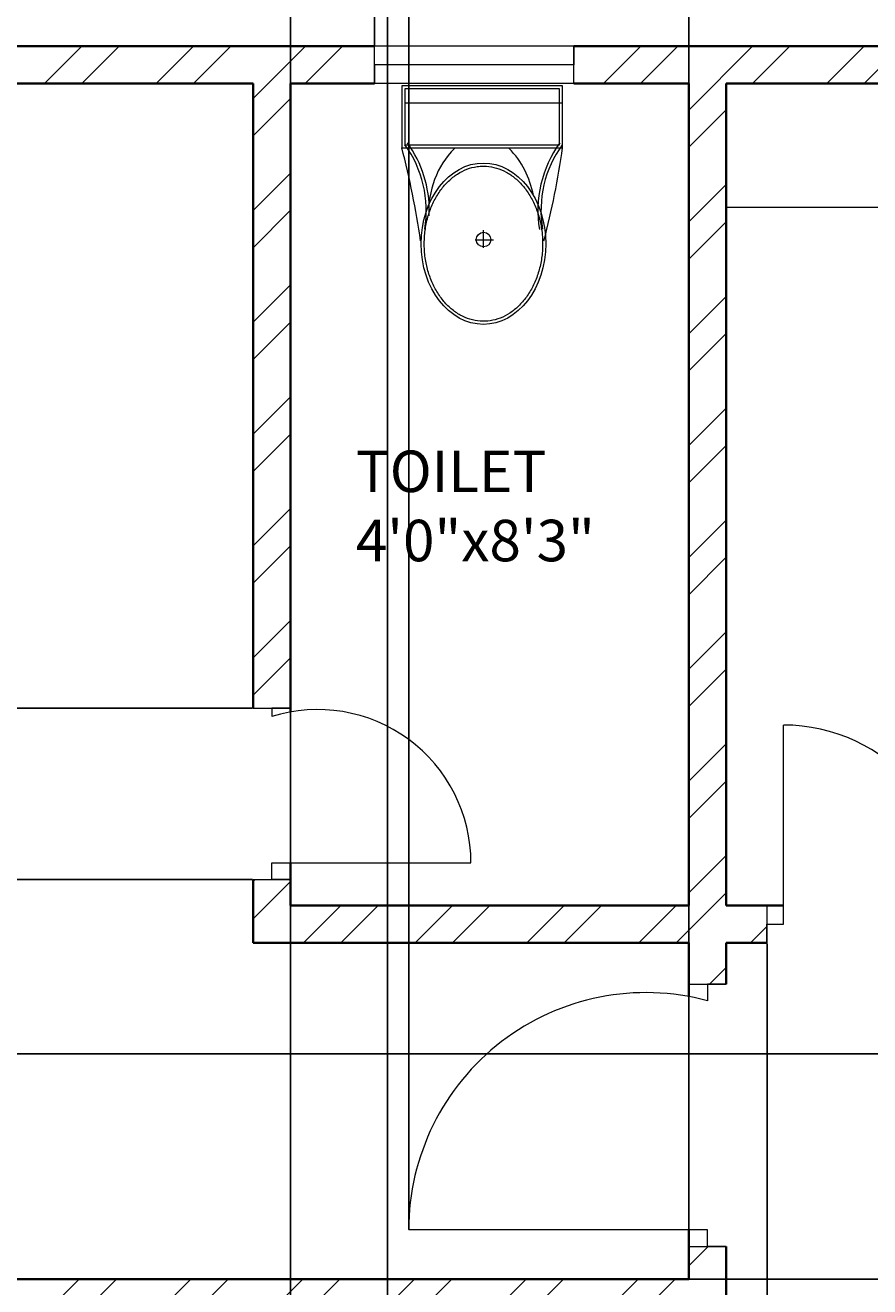
# Model space of a CAD drawing. Units: inches. Extents: x 1965 to 2673, y 1802 to 2669.
# Tile 10 of 16: x 2168 to 2270, y 2416 to 2568. Entities that reach past the tile are written whole.
import ezdxf

# ---------------------------------------------------------------- set-up
doc = ezdxf.new("R2010")
doc.units = ezdxf.units.IN
for name, color, linetype, lineweight in [('A-ANNO-DIMS', 2, 'Continuous', 18), ('A-AREA-IDEN', 7, 'Continuous', 18), ('A-DOOR', 11, 'Continuous', 18), ('A-FLOR-CASE', 8, 'Continuous', 18), ('A-FLOR-FIXT', 9, 'Continuous', 18), ('A-GLAZ', 181, 'Continuous', 18), ('A-WALL', 7, 'Continuous', 35), ('A-WALL-PATT', 252, 'Continuous', 13)]:
    doc.layers.add(name, color=color, linetype=linetype, lineweight=lineweight)
doc.styles.get("Standard").update_dxf_attribs({"font": 'arial.ttf'})
doc.dimstyles.get("Standard").update_dxf_attribs({"dimtxt": 0.18, "dimasz": 0.18, "dimexe": 0.18, "dimexo": 0.0625, "dimgap": 0.09, "dimtad": 0, "dimtih": 1, "dimtoh": 1, "dimdec": 4, "dimzin": 0, "dimdsep": 46, "dimtxsty": 'Standard', "dimcen": 0.09, "dimadec": 0, "dimazin": 0, "dimtfac": 1, "dimtdec": 4, "dimtofl": 0, "dimtmove": 0, "dimatfit": 3, "dimfxl": 1, "dimtolj": 1, "dimtzin": 0, "dimarcsym": 0})

# ---------------------------------------------------------------- blocks, each defined once
blk = doc.blocks.new('A$C31115884')
for p, q in [((283.1, 497.7), (223.4, 497.7)), ((257.5, 466.4), (257.5, 523.2)), ((0, 200), (0, 0)), ((520, 200), (0, 200)), ((10, 190), (10, 10)), ((510, 190), (10, 190)), ((510, 10), (510, 190)), ((520, 0), (520, 200)), ((510, 54.5), (0, 54.5)), ((10, 10), (510, 10)), ((0, 0), (520, 0))]:
    blk.add_line(p, q)
blk.add_circle((255.6, 496.4), 23.6)
for centre, radius, start, end in [((2777.7, -204.6), 2807, 165.4549, 171.7133), ((3237, 905), 2807, 188.2867, 194.5451), ((-294.5, 403.3), 364.7, 324.2091, 9.3499), ((-294.5, 403.3), 374.7, 324.2091, 9.3499), ((805.8, 403.3), 364.7, 170.6501, 215.7909), ((139.5, 406.2), 293.5, 315.8436, 2.6563), ((805.8, 403.3), 374.7, 179.2036, 215.7909), ((383.6, 406.2), 293.5, 190.2774, 224.1564)]:
    blk.add_arc(centre, radius, start, end)
blk.add_ellipse((256.2, 509.9), major_axis=(0, -260.7), ratio=0.772727)
blk.add_open_spline([(256.2, 259.2), (263.1, 259.2), (270, 259.7), (287.8, 262.3), (298.7, 265.1), (319.9, 273.1), (330.2, 278.4), (350.1, 291.1), (359.7, 298.7), (377.7, 315.9), (386.2, 325.5), (401.7, 346.6), (408.8, 358.1), (421.3, 382.5), (426.8, 395.5), (435.9, 422.4), (439.5, 436.4), (444.8, 465.1), (446.5, 479.7), (447.9, 509.2), (447.6, 524), (445, 553.3), (442.7, 567.8), (436.3, 596), (432.1, 609.7), (421.9, 636), (416, 648.6), (402.5, 672.1), (395, 683), (378.6, 703), (369.8, 712.1), (351.1, 728), (341.3, 734.8), (320.9, 746.2), (310.4, 750.7), (288.9, 757.3), (278, 759.4), (256, 761), (245, 760.6), (223.1, 757.2), (212.3, 754.3), (191.1, 746.1), (180.8, 740.7), (160.9, 727.8), (151.4, 720.1), (133.5, 702.7), (125.1, 693), (109.6, 671.7), (102.6, 660.2), (90.2, 635.7), (84.9, 622.7), (76, 595.6), (72.4, 581.6), (67.2, 552.9), (65.6, 538.2), (64.4, 508.8), (64.8, 494), (67.5, 464.7), (69.9, 450.2), (76.6, 422), (80.8, 408.3), (91.1, 382.2), (97.2, 369.7), (110.8, 346.3), (118.4, 335.4), (134.8, 315.6), (143.7, 306.7), (162.4, 290.9), (172.3, 284.2), (192.8, 273), (203.3, 268.6), (224.8, 262.2), (235.8, 260.2), (249.9, 259.3), (253, 259.2), (256.2, 259.2)], degree=3, knots=[0, 0, 0, 0, 0.110105, 0.110105, 0.285049, 0.285049, 0.459994, 0.459994, 0.634938, 0.634938, 0.809882, 0.809882, 0.984827, 0.984827, 1.159771, 1.159771, 1.334715, 1.334715, 1.50966, 1.50966, 1.684604, 1.684604, 1.859549, 1.859549, 2.034493, 2.034493, 2.209437, 2.209437, 2.384382, 2.384382, 2.559326, 2.559326, 2.73427, 2.73427, 2.909215, 2.909215, 3.084159, 3.084159, 3.259103, 3.259103, 3.434048, 3.434048, 3.608992, 3.608992, 3.783936, 3.783936, 3.958881, 3.958881, 4.133825, 4.133825, 4.30877, 4.30877, 4.483714, 4.483714, 4.658658, 4.658658, 4.833603, 4.833603, 5.008547, 5.008547, 5.183491, 5.183491, 5.358436, 5.358436, 5.53338, 5.53338, 5.708324, 5.708324, 5.883269, 5.883269, 6.058213, 6.058213, 6.233158, 6.233158, 6.283185, 6.283185, 6.283185, 6.283185])
blk = doc.blocks.new('WIN-24IN')
for p, q in [((0, 24), (4.5, 24)), ((0, 24), (0, 0)), ((4.5, 24), (2.25, 24)), ((2.25, 24), (2.25, 0)), ((4.5, 24), (4.5, 0)), ((2.25, 0), (0, 0)), ((0, 0), (4.5, 0))]:
    blk.add_line(p, q)
blk = doc.blocks.new('*D28')
at = {"layer": 'A-ANNO-DIMS', "color": 0, "lineweight": -2, "transparency": 16777216}
for p, q in [((2076.76, 2565.65), (2076.76, 2600.5)), ((2076.94, 2600.32), (2143.04, 2600.32)), ((2210.05, 2600.32), (2143.95, 2600.32)), ((2210.23, 2565.65), (2210.23, 2600.5))]:
    blk.add_line(p, q, dxfattribs=at)
at = {"layer": 'A-ANNO-DIMS', "color": 0, "transparency": 16777216}
for points in [[(2076.94, 2600.35), (2076.94, 2600.29), (2076.76, 2600.32)], [(2210.05, 2600.35), (2210.05, 2600.29), (2210.23, 2600.32)]]:
    blk.add_solid(points, dxfattribs=at)
at = {"layer": 'Defpoints', "color": 0, "transparency": 16777216}
for p in [(2210.23, 2600.32), (2076.76, 2565.59), (2210.23, 2565.59)]:
    blk.add_point(p, dxfattribs=at)
at = {"layer": 'A-ANNO-DIMS', "color": 0, "transparency": 16777216, "insert": (2143.49, 2600.32), "char_height": 0.18, "attachment_point": 5}
blk.add_mtext('\\A1;133.48', dxfattribs=at)
blk = doc.blocks.new('*D29')
at = {"layer": 'A-ANNO-DIMS', "color": 0, "lineweight": -2, "transparency": 16777216}
for p, q in [((2210.23, 2565.65), (2210.23, 2600.5)), ((2210.41, 2600.32), (2247.71, 2600.32)), ((2285.79, 2600.32), (2248.5, 2600.32)), ((2285.97, 2565.65), (2285.97, 2600.5))]:
    blk.add_line(p, q, dxfattribs=at)
at = {"layer": 'A-ANNO-DIMS', "color": 0, "transparency": 16777216}
for points in [[(2210.41, 2600.35), (2210.41, 2600.29), (2210.23, 2600.32)], [(2285.79, 2600.35), (2285.79, 2600.29), (2285.97, 2600.32)]]:
    blk.add_solid(points, dxfattribs=at)
at = {"layer": 'Defpoints', "color": 0, "transparency": 16777216}
for p in [(2285.97, 2600.32), (2210.23, 2565.59), (2285.97, 2565.59)]:
    blk.add_point(p, dxfattribs=at)
at = {"layer": 'A-ANNO-DIMS', "color": 0, "transparency": 16777216, "insert": (2248.1, 2600.32), "char_height": 0.18, "attachment_point": 5}
blk.add_mtext('\\A1;75.74', dxfattribs=at)
blk = doc.blocks.new('*D40')
at = {"layer": 'A-ANNO-DIMS', "color": 0, "lineweight": -2, "transparency": 16777216}
for p, q in [((2200.09, 1936.15), (2200.09, 2600.5)), ((2200.27, 2600.32), (2205.48, 2600.32)), ((2211.59, 2600.32), (2206.38, 2600.32)), ((2211.77, 1936.15), (2211.77, 2600.5))]:
    blk.add_line(p, q, dxfattribs=at)
at = {"layer": 'A-ANNO-DIMS', "color": 0, "transparency": 16777216}
for points in [[(2200.27, 2600.35), (2200.27, 2600.29), (2200.09, 2600.32)], [(2211.59, 2600.35), (2211.59, 2600.29), (2211.77, 2600.32)]]:
    blk.add_solid(points, dxfattribs=at)
at = {"layer": 'Defpoints', "color": 0, "transparency": 16777216}
for p in [(2211.77, 2600.32), (2200.09, 1936.09), (2211.77, 1936.09)]:
    blk.add_point(p, dxfattribs=at)
at = {"layer": 'A-ANNO-DIMS', "color": 0, "transparency": 16777216, "insert": (2205.93, 2600.32), "char_height": 0.18, "attachment_point": 5}
blk.add_mtext('\\A1;11.674', dxfattribs=at)
blk = doc.blocks.new('*D49')
at = {"layer": 'A-ANNO-DIMS', "color": 0, "lineweight": -2, "transparency": 16777216}
for p, q in [((2573.53, 2444.23), (2012.19, 2444.23)), ((2012.37, 2444.05), (2012.37, 2430.84)), ((2012.37, 2417.27), (2012.37, 2430.48)), ((2573.53, 2417.09), (2012.19, 2417.09))]:
    blk.add_line(p, q, dxfattribs=at)
at = {"layer": 'A-ANNO-DIMS', "color": 0, "transparency": 16777216}
for points in [[(2012.34, 2444.05), (2012.4, 2444.05), (2012.37, 2444.23)], [(2012.34, 2417.27), (2012.4, 2417.27), (2012.37, 2417.09)]]:
    blk.add_solid(points, dxfattribs=at)
at = {"layer": 'Defpoints', "color": 0, "transparency": 16777216}
for p in [(2012.37, 2444.23), (2573.59, 2444.23), (2573.59, 2417.09)]:
    blk.add_point(p, dxfattribs=at)
at = {"layer": 'A-ANNO-DIMS', "color": 0, "transparency": 16777216, "insert": (2012.37, 2430.66), "char_height": 0.18, "attachment_point": 5}
blk.add_mtext('\\A1;27.137', dxfattribs=at)
blk = doc.blocks.new('*D52')
at = {"layer": 'A-ANNO-DIMS', "color": 0, "lineweight": -2, "transparency": 16777216}
for p, q in [((2214.34, 2423.1), (2214.34, 2600.5)), ((2214.52, 2600.32), (2230.82, 2600.32)), ((2247.91, 2600.32), (2231.61, 2600.32)), ((2248.09, 2423.1), (2248.09, 2600.5))]:
    blk.add_line(p, q, dxfattribs=at)
at = {"layer": 'A-ANNO-DIMS', "color": 0, "transparency": 16777216}
for points in [[(2214.52, 2600.35), (2214.52, 2600.29), (2214.34, 2600.32)], [(2247.91, 2600.35), (2247.91, 2600.29), (2248.09, 2600.32)]]:
    blk.add_solid(points, dxfattribs=at)
at = {"layer": 'Defpoints', "color": 0, "transparency": 16777216}
for p in [(2248.09, 2600.32), (2214.34, 2423.04), (2248.09, 2423.04)]:
    blk.add_point(p, dxfattribs=at)
at = {"layer": 'A-ANNO-DIMS', "color": 0, "transparency": 16777216, "insert": (2231.22, 2600.32), "char_height": 0.18, "attachment_point": 5}
blk.add_mtext('\\A1;33.75', dxfattribs=at)
blk = doc.blocks.new('*D53')
at = {"layer": 'A-ANNO-DIMS', "color": 0, "lineweight": -2, "transparency": 16777216}
for p, q in [((2257.52, 2457.53), (2257.52, 1838.49)), ((2281.66, 2457.53), (2281.66, 1838.49)), ((2257.7, 1838.67), (2269.12, 1838.67)), ((2281.48, 1838.67), (2270.05, 1838.67))]:
    blk.add_line(p, q, dxfattribs=at)
at = {"layer": 'A-ANNO-DIMS', "color": 0, "transparency": 16777216}
for points in [[(2257.7, 1838.7), (2257.7, 1838.64), (2257.52, 1838.67)], [(2281.48, 1838.7), (2281.48, 1838.64), (2281.66, 1838.67)]]:
    blk.add_solid(points, dxfattribs=at)
at = {"layer": 'Defpoints', "color": 0, "transparency": 16777216}
for p in [(2257.52, 2457.59), (2281.66, 2457.59), (2281.66, 1838.67)]:
    blk.add_point(p, dxfattribs=at)
at = {"layer": 'A-ANNO-DIMS', "color": 0, "transparency": 16777216, "insert": (2269.59, 1838.67), "char_height": 0.18, "attachment_point": 5}
blk.add_mtext('\\A1;24.145', dxfattribs=at)
blk = doc.blocks.new('*D54')
at = {"layer": 'A-ANNO-DIMS', "color": 0, "lineweight": -2, "transparency": 16777216}
for p, q in [((2195.53, 2485.86), (2012.19, 2485.86)), ((2012.37, 2485.68), (2012.37, 2475.73)), ((2012.37, 2465.42), (2012.37, 2475.37)), ((2195.53, 2465.24), (2012.19, 2465.24))]:
    blk.add_line(p, q, dxfattribs=at)
at = {"layer": 'A-ANNO-DIMS', "color": 0, "transparency": 16777216}
for points in [[(2012.34, 2485.68), (2012.4, 2485.68), (2012.37, 2485.86)], [(2012.34, 2465.42), (2012.4, 2465.42), (2012.37, 2465.24)]]:
    blk.add_solid(points, dxfattribs=at)
at = {"layer": 'Defpoints', "color": 0, "transparency": 16777216}
for p in [(2012.37, 2485.86), (2195.59, 2485.86), (2195.59, 2465.24)]:
    blk.add_point(p, dxfattribs=at)
at = {"layer": 'A-ANNO-DIMS', "color": 0, "transparency": 16777216, "insert": (2012.37, 2475.55), "char_height": 0.18, "attachment_point": 5}
blk.add_mtext('\\A1;20.625', dxfattribs=at)

msp = doc.modelspace()

# ---------------------------------------------------------------- hatches: boundary and pattern name
at = {"layer": 'A-WALL-PATT'}
h = msp.add_hatch(dxfattribs=at)
h.set_pattern_fill('ANSI32', color=256)
h.paths.add_polyline_path([(2051.5927, 2561.0914), (2076.7559, 2561.0914), (2076.7559, 2563.3414), (2076.7559, 2565.5914), (2047.0927, 2565.5914), (2047.0927, 2518.3824), (2051.5927, 2518.3824)])
h.paths.add_polyline_path([(2051.5927, 2458.3824), (2049.3427, 2458.3824), (2047.0927, 2458.3824), (2047.0927, 2412.5914), (2248.0927, 2412.5914), (2248.0927, 2268.5914), (2252.5927, 2268.5914), (2252.5927, 2412.5914), (2252.5927, 2421.0404), (2250.3427, 2421.0404), (2248.0927, 2421.0404), (2248.0927, 2417.0914), (2051.5927, 2417.0914)])
h.paths.add_polyline_path([(2211.4933, 2268.5914), (2104.0927, 2268.5914), (2104.0927, 2272.4654), (2101.8427, 2272.4654), (2099.5927, 2272.4654), (2099.5927, 2268.5914), (2051.5927, 2268.5914), (2051.5927, 2264.0914), (2147.5927, 2264.0914), (2147.5927, 2259.8893), (2152.0927, 2259.8893), (2152.0927, 2264.0914), (2211.4933, 2264.0914), (2211.4933, 2266.3414)])
h.paths.add_polyline_path([(2104.0927, 2376.0914), (2099.5927, 2376.0914), (2047.0927, 2376.0914), (2047.0927, 2333.0682), (2051.5927, 2333.0682), (2051.5927, 2371.5914), (2099.5927, 2371.5914), (2099.5927, 2293.6123), (2104.0927, 2293.6123)], flags=17)
h.paths.add_polyline_path([(2051.5927, 2309.0682), (2047.0927, 2309.0682), (2047.0927, 2233.5821), (2051.5927, 2233.5821)])
h.paths.add_polyline_path([(2104.0927, 2412.5914), (2099.5927, 2412.5914), (2099.5927, 2376.0914), (2104.0927, 2376.0914)], flags=17)
h.paths.add_polyline_path([(2290.1254, 2268.5914), (2242.4924, 2268.5914), (2242.4924, 2264.0914), (2290.1254, 2264.0914), (2290.1254, 2266.3414)])
h.paths.add_polyline_path([(2284.653, 2264.0914), (2280.153, 2264.0914), (2280.153, 2161.6826), (2284.653, 2161.6826)])
h.paths.add_polyline_path([(2578.0927, 2329.4656), (2573.5927, 2329.4656), (2573.5927, 2268.5914), (2525.5927, 2268.5914), (2525.5927, 2271.9222), (2523.3427, 2271.9222), (2521.0927, 2271.9222), (2521.0927, 2268.5914), (2324.2835, 2268.5914), (2324.2835, 2264.0914), (2329.0927, 2264.0914), (2329.0927, 2259.4977), (2333.5927, 2259.4977), (2333.5927, 2264.0914), (2473.0927, 2264.0914), (2473.0927, 2259.9371), (2477.5927, 2259.9371), (2477.5927, 2264.0914), (2573.5927, 2264.0914), (2573.5927, 2235.5751), (2578.0927, 2235.5751)])
h.paths.add_polyline_path([(2377.0927, 2412.5914), (2578.0927, 2412.5914), (2578.0927, 2444.2286), (2575.8427, 2444.2286), (2573.5927, 2444.2286), (2573.5927, 2417.0914), (2429.5927, 2417.0914), (2377.0927, 2417.0914), (2377.0927, 2421.7443), (2372.5927, 2421.7443), (2372.5927, 2268.5914), (2377.0927, 2268.5914)])
h.paths.add_polyline_path([(2525.5927, 2371.5914), (2573.5927, 2371.5914), (2573.5927, 2353.4656), (2578.0927, 2353.4656), (2578.0927, 2376.0914), (2525.5927, 2376.0914), (2521.0927, 2376.0914), (2521.0927, 2290.6472), (2525.5927, 2290.6472)], flags=17)
h.paths.add_polyline_path([(2477.5927, 2236.4106), (2475.3427, 2236.4106), (2473.0927, 2236.4106), (2473.0927, 2084.5914), (2465.3309, 2084.5914), (2465.3309, 2080.0914), (2481.6764, 2080.0914), (2481.6764, 2082.3414), (2481.6764, 2084.5914), (2477.5927, 2084.5914), (2477.5927, 2151.5914), (2573.5927, 2151.5914), (2573.5927, 2130.2907), (2578.0927, 2130.2907), (2578.0927, 2199.5751), (2575.8427, 2199.5751), (2573.5927, 2199.5751), (2573.5927, 2156.0914), (2477.5927, 2156.0914)])
h.paths.add_polyline_path([(2573.5927, 2084.5914), (2505.5513, 2084.5914), (2505.5513, 2080.0914), (2573.5927, 2080.0914)], flags=17)
h.paths.add_polyline_path([(2578.0927, 2106.2907), (2575.8427, 2106.2907), (2573.5927, 2106.2907), (2573.5927, 2050.8986), (2578.0927, 2050.8986)])
h.paths.add_polyline_path([(2578.0927, 1990.8986), (2575.8427, 1990.8986), (2573.5927, 1990.8986), (2573.5927, 1936.0914), (2522.132, 1936.0914), (2522.132, 1931.5914), (2578.0927, 1931.5914)])
h.paths.add_polyline_path([(2462.132, 1936.0914), (2429.5927, 1936.0914), (2429.5927, 2080.0914), (2432.623, 2080.0914), (2432.623, 2082.3414), (2432.623, 2084.5914), (2429.5927, 2084.5914), (2429.5927, 2120.5914), (2333.5927, 2120.5914), (2333.5927, 2229.3125), (2331.3427, 2229.3125), (2329.0927, 2229.3125), (2329.0927, 2116.0914), (2425.0927, 2116.0914), (2425.0927, 1936.0914), (2346.4058, 1936.0914), (2346.4058, 1931.5914), (2462.132, 1931.5914), (2462.132, 1933.8414)])
h.paths.add_polyline_path([(2211.767, 1933.8414), (2211.767, 1936.0914), (2200.0927, 1936.0914), (2200.0927, 2080.0914), (2200.0927, 2116.0914), (2284.653, 2116.0914), (2284.653, 2130.591), (2282.403, 2130.591), (2280.153, 2130.591), (2280.153, 2120.5914), (2200.0927, 2120.5914), (2195.5927, 2120.5914), (2195.5927, 2080.0914), (2195.5927, 1936.0914), (2139.0533, 1936.0914), (2139.0533, 1931.5914), (2211.767, 1931.5914)])
h.paths.add_polyline_path([(2282.2502, 1933.8414), (2282.2502, 1936.0914), (2259.767, 1936.0914), (2259.767, 1931.5914), (2282.2502, 1931.5914)], flags=17)
h.paths.add_polyline_path([(2051.5927, 1987.096), (2049.3427, 1987.096), (2047.0927, 1987.096), (2047.0927, 1931.5914), (2079.0533, 1931.5914), (2079.0533, 1933.8414), (2079.0533, 1936.0914), (2051.5927, 1936.0914)])
h.paths.add_polyline_path([(2051.5927, 2197.5821), (2049.3427, 2197.5821), (2047.0927, 2197.5821), (2047.0927, 2141.952), (2051.5927, 2141.952), (2051.5927, 2151.5914), (2147.5927, 2151.5914), (2147.5927, 2084.5914), (2144.3652, 2084.5914), (2144.3652, 2080.0914), (2155.9662, 2080.0914), (2155.9662, 2082.3414), (2155.9662, 2084.5914), (2152.0927, 2084.5914), (2152.0927, 2239.4921), (2149.8427, 2239.4921), (2147.5927, 2239.4921), (2147.5927, 2156.0914), (2051.5927, 2156.0914)])
h.paths.add_polyline_path([(2051.5927, 2080.0914), (2123.8575, 2080.0914), (2123.8575, 2082.3414), (2123.8575, 2084.5914), (2051.5927, 2084.5914), (2051.5927, 2117.952), (2047.0927, 2117.952), (2047.0927, 2047.096), (2051.5927, 2047.096)])
h = msp.add_hatch(dxfattribs=at)
h.set_pattern_fill('ANSI32', color=256)
h.paths.add_polyline_path([(2210.2316, 2563.3414), (2210.2316, 2565.5914), (2136.7559, 2565.5914), (2136.7559, 2561.0914), (2195.5927, 2561.0914), (2195.5927, 2485.8604), (2200.0927, 2485.8604), (2200.0927, 2561.0914), (2210.2316, 2561.0914)])
h.paths.add_polyline_path([(2285.9734, 2565.5914), (2234.2316, 2565.5914), (2234.2316, 2561.0914), (2248.0927, 2561.0914), (2248.0927, 2462.0914), (2200.0927, 2462.0914), (2200.0927, 2465.2357), (2197.8427, 2465.2357), (2195.5927, 2465.2357), (2195.5927, 2457.5914), (2248.0927, 2457.5914), (2248.0927, 2452.628), (2252.5927, 2452.628), (2252.5927, 2457.5914), (2257.5156, 2457.5914), (2257.5156, 2459.8414), (2257.5156, 2462.0914), (2252.5927, 2462.0914), (2252.5927, 2561.0914), (2285.9734, 2561.0914)])
h.paths.add_polyline_path([(2213.1374, 1872.8885), (2461.061, 1872.8885), (2461.061, 1909.9813), (2213.1374, 1909.9813)], flags=9)
h.paths.add_polyline_path([(2328.4056, 1942.3944), (2340.6089, 1942.3944), (2340.6089, 1952.6979), (2328.4056, 1952.6979)], flags=9)
h.paths.add_polyline_path([(2353.5759, 2030.9808), (2376.6455, 2030.9808), (2376.6455, 2041.2844), (2353.5759, 2041.2844)], flags=9)
h.paths.add_polyline_path([(2289.989, 2074.1041), (2326.916, 2074.1041), (2326.916, 2092.7615), (2289.989, 2092.7615)], flags=9)
h.paths.add_polyline_path([(2497.9, 2052.8638), (2548.3741, 2052.8638), (2548.3741, 2071.5212), (2497.9, 2071.5212)], flags=9)
h.paths.add_polyline_path([(2486.59, 2116.4883), (2515.7475, 2116.4883), (2515.7475, 2135.1456), (2486.59, 2135.1456)], flags=9)
h.paths.add_polyline_path([(2497.3007, 2181.2877), (2530.459, 2181.2877), (2530.459, 2199.945), (2497.3007, 2199.945)], flags=9)
h.paths.add_polyline_path([(2288.237, 2190.3228), (2324.1238, 2190.3228), (2324.1238, 2208.9802), (2288.237, 2208.9802)], flags=9)
h.paths.add_polyline_path([(2350.806, 2127.8307), (2387.733, 2127.8307), (2387.733, 2146.488), (2350.806, 2146.488)], flags=9)
h.paths.add_polyline_path([(2530.3237, 2315.2679), (2559.5563, 2315.2679), (2559.5563, 2333.9252), (2530.3237, 2333.9252)], flags=9)
h.paths.add_polyline_path([(2418.419, 2383.4707), (2468.2894, 2383.4707), (2468.2894, 2402.1281), (2418.419, 2402.1281)], flags=9)
h.paths.add_polyline_path([(2327.4503, 2399.0281), (2364.3773, 2399.0281), (2364.3773, 2417.6854), (2327.4503, 2417.6854)], flags=9)
h.paths.add_polyline_path([(2147.9722, 2271.4601), (2197.8426, 2271.4601), (2197.8426, 2290.1174), (2147.9722, 2290.1174)], flags=9)
h.paths.add_polyline_path([(2474.3875, 2421.594), (2524.8616, 2421.594), (2524.8616, 2440.2514), (2474.3875, 2440.2514)], flags=9)
h.paths.add_polyline_path([(2063.9863, 2052.9059), (2114.4604, 2052.9059), (2114.4604, 2071.5632), (2063.9863, 2071.5632)], flags=9)
h.paths.add_polyline_path([(2200.3335, 2133.7067), (2237.2605, 2133.7067), (2237.2605, 2152.364), (2200.3335, 2152.364)], flags=9)
h.paths.add_polyline_path([(2080.5973, 2184.636), (2113.8681, 2184.636), (2113.8681, 2203.2933), (2080.5973, 2203.2933)], flags=9)
h.paths.add_polyline_path([(2102.4918, 2116.4497), (2131.6494, 2116.4497), (2131.6494, 2135.107), (2102.4918, 2135.107)], flags=9)
h.paths.add_polyline_path([(2056.2753, 2308.5576), (2085.5079, 2308.5576), (2085.5079, 2327.2149), (2056.2753, 2327.2149)], flags=9)
h.paths.add_polyline_path([(2385.619, 2500.9729), (2414.8516, 2500.9729), (2414.8516, 2519.6303), (2385.619, 2519.6303)], flags=9)
h.paths.add_polyline_path([(2286.6643, 2508.6826), (2320.0715, 2508.6826), (2320.0715, 2527.34), (2286.6643, 2527.34)], flags=9)
h.paths.add_polyline_path([(2206.5604, 2500.7243), (2235.793, 2500.7243), (2235.793, 2519.3817), (2206.5604, 2519.3817)], flags=25)
h.paths.add_polyline_path([(2062.6644, 2424.4027), (2112.5348, 2424.4027), (2112.5348, 2443.0601), (2062.6644, 2443.0601)], flags=9)
h = msp.add_hatch(dxfattribs=at)
h.set_pattern_fill('ANSI32', color=256)
h.paths.add_polyline_path([(2429.5927, 2468.6101), (2427.3427, 2468.6101), (2425.0927, 2468.6101), (2425.0927, 2462.0914), (2377.0927, 2462.0914), (2377.0927, 2561.0914), (2390.4173, 2561.0914), (2390.4173, 2565.5914), (2321.9734, 2565.5914), (2321.9734, 2561.0914), (2372.5927, 2561.0914), (2372.5927, 2462.0914), (2281.6605, 2462.0914), (2281.6605, 2457.5914), (2372.5927, 2457.5914), (2372.5927, 2451.3316), (2377.0927, 2451.3316), (2377.0927, 2457.5914), (2429.5927, 2457.5914)])
h.paths.add_polyline_path([(2480.8929, 2565.5914), (2414.4173, 2565.5914), (2414.4173, 2561.0914), (2425.0927, 2561.0914), (2425.0927, 2489.9153), (2429.5927, 2489.9153), (2429.5927, 2561.0914), (2480.8929, 2561.0914), (2480.8929, 2563.3414)])
h.paths.add_polyline_path([(2213.1374, 1872.8885), (2461.061, 1872.8885), (2461.061, 1909.9813), (2213.1374, 1909.9813)], flags=9)
h.paths.add_polyline_path([(2328.4056, 1942.3944), (2340.6089, 1942.3944), (2340.6089, 1952.6979), (2328.4056, 1952.6979)], flags=9)
h.paths.add_polyline_path([(2353.5759, 2030.9808), (2376.6455, 2030.9808), (2376.6455, 2041.2844), (2353.5759, 2041.2844)], flags=9)
h.paths.add_polyline_path([(2289.989, 2074.1041), (2326.916, 2074.1041), (2326.916, 2092.7615), (2289.989, 2092.7615)], flags=9)
h.paths.add_polyline_path([(2497.9, 2052.8638), (2548.3741, 2052.8638), (2548.3741, 2071.5212), (2497.9, 2071.5212)], flags=9)
h.paths.add_polyline_path([(2486.59, 2116.4883), (2515.7475, 2116.4883), (2515.7475, 2135.1456), (2486.59, 2135.1456)], flags=9)
h.paths.add_polyline_path([(2497.3007, 2181.2877), (2530.459, 2181.2877), (2530.459, 2199.945), (2497.3007, 2199.945)], flags=9)
h.paths.add_polyline_path([(2288.237, 2190.3228), (2324.1238, 2190.3228), (2324.1238, 2208.9802), (2288.237, 2208.9802)], flags=9)
h.paths.add_polyline_path([(2350.806, 2127.8307), (2387.733, 2127.8307), (2387.733, 2146.488), (2350.806, 2146.488)], flags=9)
h.paths.add_polyline_path([(2530.3237, 2315.2679), (2559.5563, 2315.2679), (2559.5563, 2333.9252), (2530.3237, 2333.9252)], flags=9)
h.paths.add_polyline_path([(2418.419, 2383.4707), (2468.2894, 2383.4707), (2468.2894, 2402.1281), (2418.419, 2402.1281)], flags=9)
h.paths.add_polyline_path([(2327.4503, 2399.0281), (2364.3773, 2399.0281), (2364.3773, 2417.6854), (2327.4503, 2417.6854)], flags=9)
h.paths.add_polyline_path([(2147.9722, 2271.4601), (2197.8426, 2271.4601), (2197.8426, 2290.1174), (2147.9722, 2290.1174)], flags=9)
h.paths.add_polyline_path([(2474.3875, 2421.594), (2524.8616, 2421.594), (2524.8616, 2440.2514), (2474.3875, 2440.2514)], flags=9)
h.paths.add_polyline_path([(2063.9863, 2052.9059), (2114.4604, 2052.9059), (2114.4604, 2071.5632), (2063.9863, 2071.5632)], flags=9)
h.paths.add_polyline_path([(2200.3335, 2133.7067), (2237.2605, 2133.7067), (2237.2605, 2152.364), (2200.3335, 2152.364)], flags=9)
h.paths.add_polyline_path([(2080.5973, 2184.636), (2113.8681, 2184.636), (2113.8681, 2203.2933), (2080.5973, 2203.2933)], flags=9)
h.paths.add_polyline_path([(2102.4918, 2116.4497), (2131.6494, 2116.4497), (2131.6494, 2135.107), (2102.4918, 2135.107)], flags=9)
h.paths.add_polyline_path([(2056.2753, 2308.5576), (2085.5079, 2308.5576), (2085.5079, 2327.2149), (2056.2753, 2327.2149)], flags=9)
h.paths.add_polyline_path([(2385.619, 2500.9729), (2414.8516, 2500.9729), (2414.8516, 2519.6303), (2385.619, 2519.6303)], flags=25)
h.paths.add_polyline_path([(2286.6643, 2508.6826), (2320.0715, 2508.6826), (2320.0715, 2527.34), (2286.6643, 2527.34)], flags=25)
h.paths.add_polyline_path([(2206.5604, 2500.7243), (2235.793, 2500.7243), (2235.793, 2519.3817), (2206.5604, 2519.3817)], flags=9)
h.paths.add_polyline_path([(2062.6644, 2424.4027), (2112.5348, 2424.4027), (2112.5348, 2443.0601), (2062.6644, 2443.0601)], flags=9)

# ---------------------------------------------------------------- linework, layer by layer
at = {"layer": 'A-DOOR'}
for p, q in [((2195.5927, 2485.8604), (2200.0927, 2485.8604)), ((2200.0927, 2485.8604), (2197.8427, 2485.8604)), ((2197.8427, 2485.8604), (2197.8427, 2484.8604)), ((2259.5156, 2459.8414), (2259.5156, 2483.8414)), ((2197.8427, 2465.2357), (2197.8427, 2467.2357)), ((2197.8427, 2467.2357), (2221.8427, 2467.2357)), ((2195.5927, 2465.2357), (2200.0927, 2465.2357)), ((2200.0927, 2465.2357), (2197.8427, 2465.2357)), ((2257.5156, 2462.0914), (2257.5156, 2457.5914)), ((2257.5156, 2457.5914), (2257.5156, 2459.8414)), ((2257.5156, 2459.8414), (2259.5156, 2459.8414)), ((2248.0927, 2452.628), (2252.5927, 2452.628)), ((2252.5927, 2452.628), (2250.3427, 2452.628)), ((2250.3427, 2452.628), (2250.3427, 2450.628)), ((2250.3427, 2423.0404), (2214.3427, 2423.0404)), ((2250.3427, 2421.0404), (2250.3427, 2423.0404)), ((2248.0927, 2421.0404), (2252.5927, 2421.0404)), ((2252.5927, 2421.0404), (2250.3427, 2421.0404))]:
    msp.add_line(p, q, dxfattribs=at)
for centre, radius, start, end in [((2203.3713, 2467.2357), 18.4714, 0, 107.415746), ((2259.5156, 2463.3869), 20.4545, 350.018178, 90), ((2242.9133, 2423.0404), 28.5706, 74.927643, 180)]:
    msp.add_arc(centre, radius, start, end, dxfattribs=at)
at = {"layer": 'A-FLOR-CASE'}
msp.add_line((2252.5927, 2546.2207), (2355.5796, 2546.2207), dxfattribs=at)
at = {"layer": 'A-WALL'}
for p, q in [((2136.7559, 2565.5914), (2210.2316, 2565.5914)), ((2234.2316, 2565.5914), (2285.9734, 2565.5914)), ((2136.7559, 2561.0914), (2195.5927, 2561.0914)), ((2147.5927, 2561.0914), (2195.5927, 2561.0914)), ((2195.5927, 2561.0914), (2195.5927, 2485.8604)), ((2200.0927, 2561.0914), (2200.0927, 2485.4139)), ((2200.0927, 2561.0914), (2210.2316, 2561.0914)), ((2234.2316, 2561.0914), (2248.0927, 2561.0914)), ((2248.0927, 2561.0914), (2248.0927, 2462.0914)), ((2252.5927, 2561.0914), (2252.5927, 2462.0914)), ((2252.5927, 2561.0914), (2285.9734, 2561.0914)), ((2200.0927, 2467.2357), (2200.0927, 2462.0914)), ((2195.5927, 2465.2357), (2195.5927, 2457.5914)), ((2200.0927, 2462.0914), (2248.0927, 2462.0914)), ((2200.0927, 2462.0914), (2248.0927, 2462.0914)), ((2252.5927, 2462.0914), (2259.5156, 2462.0914)), ((2195.5927, 2457.5914), (2248.0927, 2457.5914)), ((2200.0927, 2457.5914), (2248.0927, 2457.5914)), ((2248.0927, 2457.5914), (2248.0927, 2451.1375)), ((2252.5927, 2457.5914), (2257.5156, 2457.5914)), ((2252.5927, 2457.5914), (2252.5927, 2452.628)), ((2248.0927, 2423.0404), (2248.0927, 2417.0914)), ((2252.5927, 2421.0404), (2252.5927, 2268.5914)), ((2051.5927, 2417.0914), (2248.0927, 2417.0914))]:
    msp.add_line(p, q, dxfattribs=at)

# ---------------------------------------------------------------- block references
at = {"layer": 'A-FLOR-FIXT', "xscale": 0.0372717239612423, "yscale": 0.0372717239612423, "zscale": 0.0372717239612423, "rotation": 180}
msp.add_blockref('A$C31115884', (2232.8936, 2560.815), dxfattribs=at)
at = {"layer": 'A-GLAZ', "extrusion": (0, 0, -1), "zscale": -1, "rotation": 90}
msp.add_blockref('WIN-24IN', (-2210.2359, 2561.0887), dxfattribs=at)

# ---------------------------------------------------------------- texts
at = {"layer": 'A-AREA-IDEN', "insert": (2207.9741, 2516.897), "char_height": 5, "attachment_point": 1}
msp.add_mtext_dynamic_manual_height_columns('TOILET\\P4\'0"x8\'3"', width=98.233579, gutter_width=12.5, heights=[0], dxfattribs=at)

# ---------------------------------------------------------------- dimensions: what is measured, and where the dimension line sits
at = {"layer": 'A-ANNO-DIMS'}
for base, p1, p2, override, picture, middle in [((2210.2316, 2600.3164), (2076.7559, 2565.5914), (2210.2316, 2565.5914), {"dimdec": 2, "dimlfac": 1, "dimrnd": 0, "dimzin": 0, "dimdsep": 46, "dimlunit": 2}, '*D28', (2143.4937, 2600.3164)), ((2211.767, 2600.3164), (2200.0927, 1936.0914), (2211.767, 1936.0914), {"dimdec": 3, "dimlfac": 1, "dimrnd": 0, "dimzin": 0, "dimdsep": 46, "dimlunit": 2}, '*D40', (2205.9299, 2600.3164)), ((2285.9734, 2600.3164), (2210.2316, 2565.5914), (2285.9734, 2565.5914), {"dimdec": 2, "dimlfac": 1, "dimrnd": 0, "dimzin": 0, "dimdsep": 46, "dimlunit": 2}, '*D29', (2248.1025, 2600.3164)), ((2248.0927, 2600.3164), (2214.3427, 2423.0404), (2248.0927, 2423.0404), {"dimdec": 2, "dimlfac": 1, "dimrnd": 0, "dimzin": 0, "dimdsep": 46, "dimlunit": 2}, '*D52', (2231.2177, 2600.3164)), ((2281.6605, 1838.6715), (2257.5156, 2457.5914), (2281.6605, 2457.5914), {"dimdec": 3, "dimlfac": 1, "dimrnd": 0, "dimzin": 0, "dimdsep": 46, "dimlunit": 2}, '*D53', (2269.588, 1838.6715))]:
    dim = msp.add_linear_dim(base=base, p1=p1, p2=p2, dimstyle='Standard', override=override, dxfattribs=at)
    dim.commit()
    dim.dimension.update_dxf_attribs({"geometry": picture, "text_midpoint": middle})
for base, p1, p2, picture, middle in [((2012.3677, 2485.8604), (2195.5927, 2465.2357), (2195.5927, 2485.8604), '*D54', (2012.3677, 2475.548)), ((2012.3677, 2444.2286), (2573.5927, 2417.0914), (2573.5927, 2444.2286), '*D49', (2012.3677, 2430.66))]:
    dim = msp.add_linear_dim(base=base, p1=p1, p2=p2, angle=90, dimstyle='Standard', override={"dimdec": 3, "dimlfac": 1, "dimrnd": 0, "dimzin": 0, "dimdsep": 46, "dimlunit": 2}, dxfattribs=at)
    dim.commit()
    dim.dimension.update_dxf_attribs({"geometry": picture, "text_midpoint": middle})

doc.saveas('drawing.dxf')
